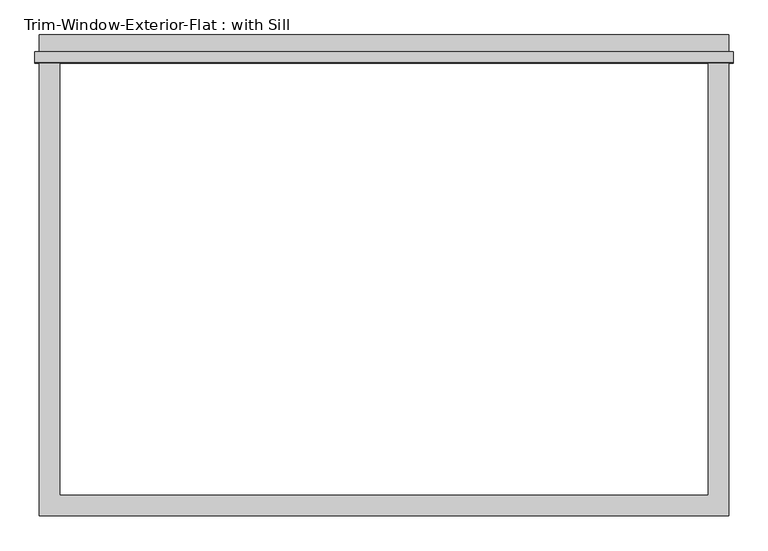
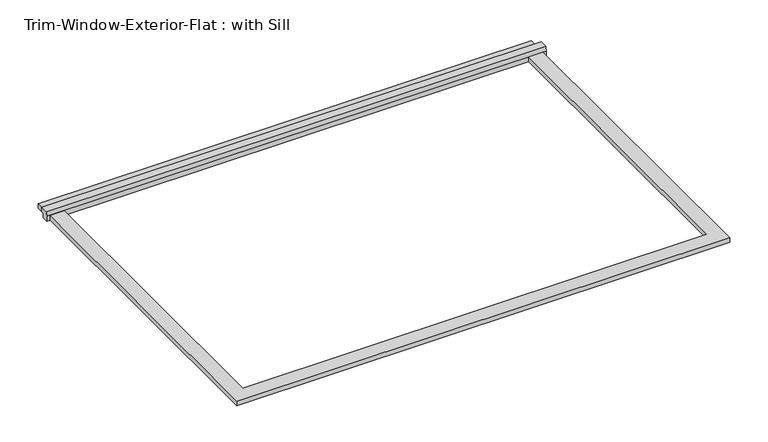
"""IFC4 building model written with IfcOpenShell, lengths in millimetres: proxy geometry, Trim-Window-Exterior-Flat : with Sill."""

from ifc_helpers import new_model, si_unit, frame, origin, origin_with_axes, place, context, project, spatial, polyline, outline, extrude, source, transform, mapped, element, save


def trim_window_exterior_flat_with_sill_db7a9870(model_context):
    return source(origin(), model_context, "Body", "SweptSolid", [
        extrude(outline(polyline([(971.55, 1241.3823709), (-971.55, 1241.3823709), (-971.55, 1298.5323709), (971.55, 1298.5323709), (971.55, 1241.3823709)])), origin_with_axes(), (0.0, 0.0, 1.0), 19.05),
        extrude(outline(polyline([(1250.95, 38.1), (1250.95, 19.05), (1241.3823709, 19.05), (1241.3823709, 0.0), (1219.2, 0.0), (1219.2, 19.05), (1221.6580645, 38.1), (1250.95, 38.1)])), frame((-984.25, 0.0, 0.0), z_axis=(1.0, 0.0, 0.0), x_axis=(0.0, 1.0, 0.0)), (0.0, 0.0, 1.0), 1968.5),
        extrude(outline(polyline([(-971.55, -57.15), (-971.55, 1219.2), (-914.4, 1219.2), (-914.4, 0.0), (914.4, 0.0), (914.4, 1219.2), (971.55, 1219.2), (971.55, -57.15), (-971.55, -57.15)])), origin_with_axes(), (0.0, 0.0, 1.0), 19.05),
    ])


if __name__ == "__main__":
    model = new_model("IFC4")
    model_context = context("Model", 3, world=origin())
    ifc_project = project(units=[si_unit("LENGTHUNIT", "METRE", prefix="MILLI")], contexts=[model_context])
    site = spatial("IfcSite", under=ifc_project)
    building = spatial("IfcBuilding", under=site)
    placement = place(None, origin())
    trim_window_exterior_flat_with_sill_shape = trim_window_exterior_flat_with_sill_db7a9870(model_context)
    element("IfcBuildingElementProxy", 1, Name="Trim-Window-Exterior-Flat : with Sill", ObjectType="Trim-Window-Exterior-Flat : with Sill", at=placement, inside=building, context=model_context, shape_type="MappedRepresentation", body=[
        mapped(trim_window_exterior_flat_with_sill_shape, transform((0.0, 0.0, 0.0), x_axis=(1.0, 0.0, 0.0), y_axis=(0.0, 1.0, 0.0), z_axis=(0.0, 0.0, 1.0))),
    ])
    save(model, "model.ifc")

# Revit data of these elements
# Type "Trim-Window-Exterior-Flat : with Sill"
#   Trim Width = 0' - 2 1/4"
#   Trim Thickness_Picture Frame = 0' - 1 1/4"
#   Trim Thickness_with Sill = 0' - 0 3/4"
#   Sill Thickness = 0' - 1 1/4"
#   Opening Width [instance default] = 2' - 0"
#   Opening Height [instance default] = 3' - 0"
#   Default Elevation = 4' - 0"
#   Sill = yes
#   Picture Frame = no
#   Trim Material [instance default] = none
# Element 1 (IfcBuildingElementProxy, "Trim-Window-Exterior-Flat : with Sill")
#   Opening Width = 6' - 0"
#   Opening Height = 4' - 0"
#   Trim Material = Clad - White
#   Materials on its faces: "Clad - White"
# Materials
#   "Clad - White": class "Wood", colour RGB 242 242 238, transparency 0, Cost = 0
